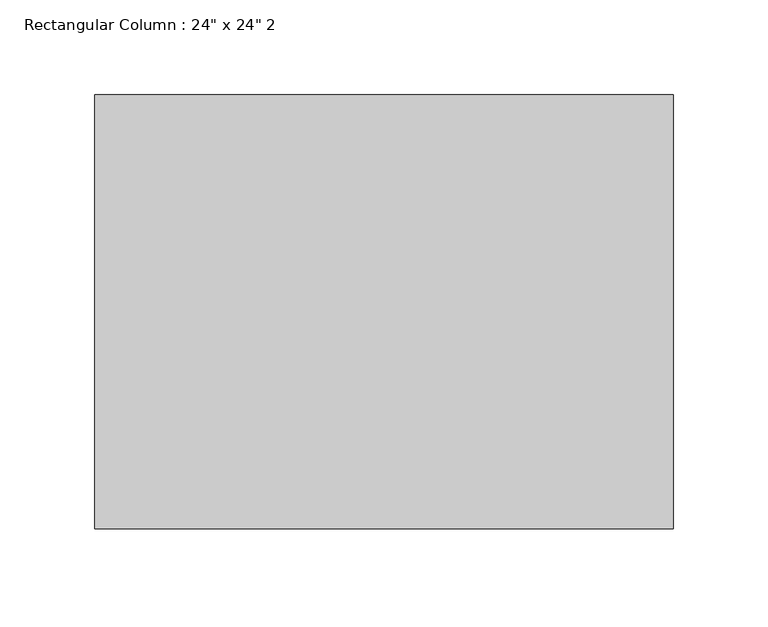
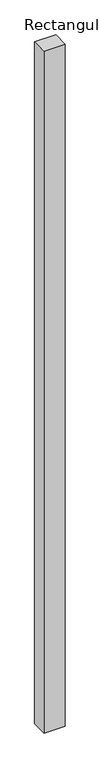
"""IFC4 building model written with IfcOpenShell, lengths in millimetres: column geometry."""

from ifc_helpers import new_model, si_unit, origin, origin_with_axes, place, context, project, spatial, polyline, outline, extrude, source, transform, mapped, element, save


def column_4e4144c7(model_context):
    return source(origin(), model_context, "Body", "SweptSolid", [
        extrude(outline(polyline([(152.4, 114.3), (152.4, -114.3), (-152.4, -114.3), (-152.4, 114.3), (152.4, 114.3)])), origin_with_axes(), (0.0, 0.0, 1.0), 10363.2),
    ])


if __name__ == "__main__":
    model = new_model("IFC4")
    model_context = context("Model", 3, world=origin())
    ifc_project = project(units=[si_unit("LENGTHUNIT", "METRE", prefix="MILLI")], contexts=[model_context])
    site = spatial("IfcSite", under=ifc_project)
    building = spatial("IfcBuilding", under=site)
    placement = place(None, origin())
    column_shape = column_4e4144c7(model_context)
    element("IfcColumn", 1, ObjectType="Rectangular Column : 24\" x 24\" 2", at=placement, inside=building, context=model_context, shape_type="MappedRepresentation", body=[
        mapped(column_shape, transform((0.0, 0.0, 0.0), x_axis=(1.0, 0.0, 0.0), y_axis=(0.0, 1.0, 0.0), z_axis=(0.0, 0.0, 1.0))),
    ])
    save(model, "model.ifc")

# Revit data of these elements
# Type "Rectangular Column : 24\" x 24\" 2"
#   Assembly Code = "B1010200"
#   Depth = 0' - 9"
#   Offset Base = 0' - 0"
#   Offset Top = 0' - 0"
#   Width = 1' - 0"
#   Material = none
